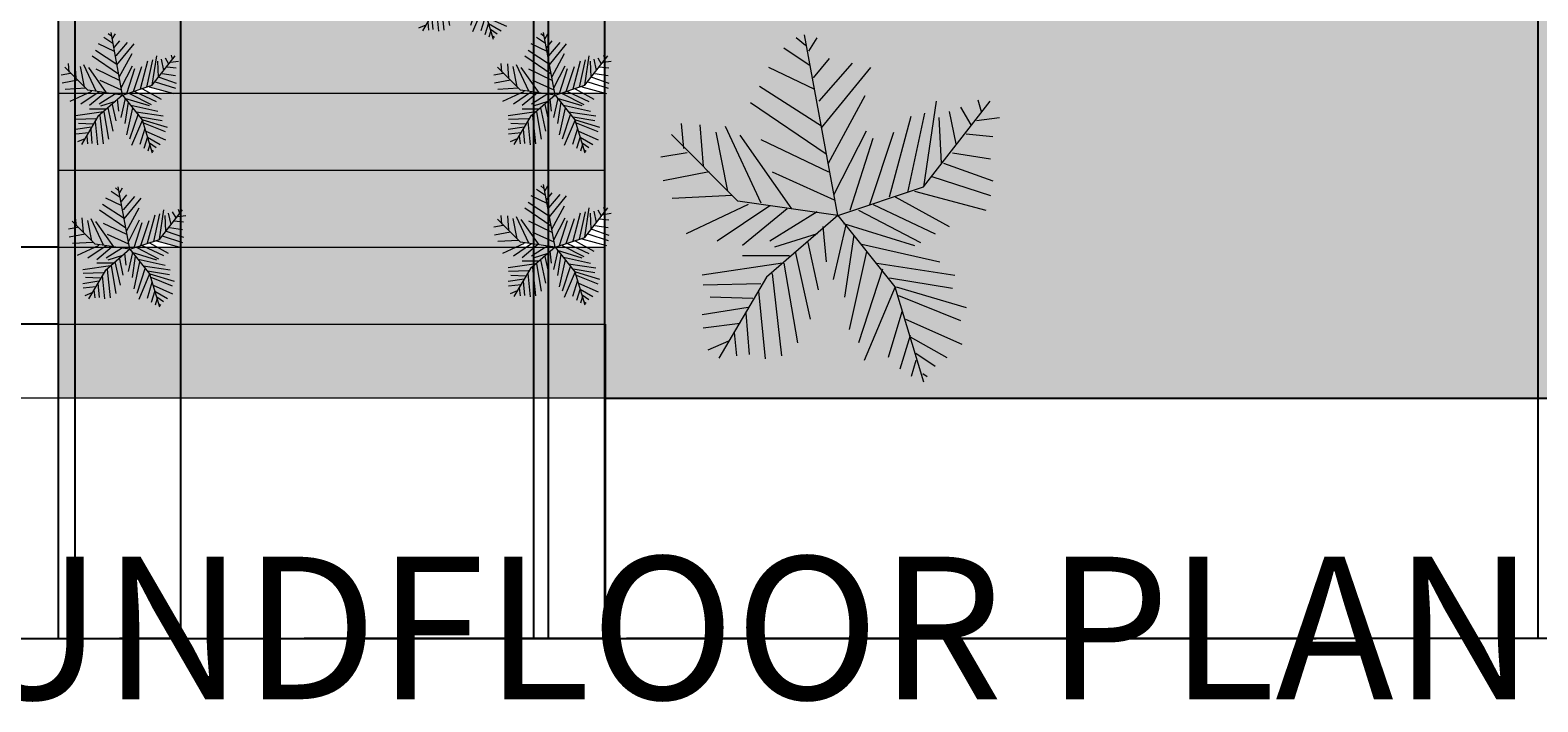
# Model space of a CAD drawing. Units: millimetres. Extents: x -229 to 16545, y -10488 to 4272.
# Tile 6 of 29: x 5862 to 12015, y -10488 to -7746. Entities that reach past the tile are written whole.
import ezdxf

# ---------------------------------------------------------------- set-up
doc = ezdxf.new("R2010")
doc.units = ezdxf.units.MM
for name, color, linetype, lineweight in [('A-ANNO-DIMS', 2, 'Continuous', 18), ('A-ANNO-TEXT', 7, 'Continuous', 25), ('A-FLOR-STRS', 7, 'Continuous', 18), ('L-PLNT-TREE', 80, 'Continuous', 18), ('L-PVMT', 7, 'Continuous', 18)]:
    doc.layers.add(name, color=color, linetype=linetype, lineweight=lineweight)
doc.layers.add('A-FLOR-STRS-PATT', color=51, linetype='Continuous', lineweight=13, true_color=0xf8f6b0)
doc.layers.add('L-PLNT-PATT', color=116, linetype='Continuous', lineweight=13, true_color=0x136734)
doc.styles.get("Standard").update_dxf_attribs({"font": 'arial.ttf'})
doc.dimstyles.get("Standard").update_dxf_attribs({"dimtxt": 0.18, "dimasz": 0.18, "dimexe": 0.18, "dimexo": 0.0625, "dimgap": 0.09, "dimtad": 0, "dimtih": 1, "dimtoh": 1, "dimdec": 4, "dimzin": 0, "dimdsep": 46, "dimtxsty": 'Standard', "dimcen": 0.09, "dimadec": 0, "dimazin": 0, "dimtfac": 1, "dimtdec": 4, "dimtofl": 0, "dimtmove": 0, "dimatfit": 3, "dimfxl": 1, "dimtolj": 1, "dimtzin": 0, "dimarcsym": 0})

# ---------------------------------------------------------------- blocks, each defined once
blk = doc.blocks.new('*U18')
for p, q in [((-8.737, 47.138), (-17.069, 52.711)), ((-10.186, 53.64), (-13.084, 55.962)), ((0, 0), (-10.5, 57)), ((-9.099, 51.782), (-6.563, 55.962)), ((-7.65, 43.423), (-2.578, 49.46)), ((-5.839, 35.992), (4.667, 48.067)), ((-7.288, 39.707), (-21.778, 46.673)), ((-5.114, 27.632), (10.463, 46.673)), ((-5.114, 28.097), (-24.676, 40.636)), ((-3.665, 19.273), (-27.574, 35.527)), ((-2.941, 16.486), (8.652, 37.85)), ((27, 9), (48, 36)), ((27.127, 9.056), (31.112, 35.992)), ((38.719, 34.134), (41.979, 28.561)), ((44.153, 36.456), (45.239, 32.741)), ((-48.585, 21.131), (-49.309, 29.026)), ((-43.513, 28.561), (-42.427, 15.558)), ((16.259, 5.805), (23.142, 31.348)), ((22.055, 7.198), (27.489, 32.277)), ((31.836, 30.883), (32.561, 16.486)), ((35.096, 32.741), (37.27, 22.524)), ((43.791, 29.954), (51.036, 30.883)), ((-31.5, 4.5), (-52.5, 25.5)), ((-38.442, 26.239), (-34.819, 7.663)), ((-35.544, 28.097), (-24.314, 3.947)), ((-14.533, 2.09), (-30.834, 25.31)), ((-24.314, 23.917), (-2.941, 13.7)), ((-1.129, 6.734), (9.014, 26.704)), ((3.942, 1.625), (11.187, 24.381)), ((10.101, 3.483), (17.708, 26.239)), ((40.53, 25.775), (48.862, 24.846)), ((-47.498, 19.737), (-55.83, 18.344)), ((36.183, 19.737), (48.137, 17.88)), ((33.285, 16.486), (48.862, 10.913)), ((-40.615, 13.7), (-55.105, 10.913)), ((-20.691, 13.7), (-1.129, 4.876)), ((29.662, 12.307), (48.137, 6.269)), ((-33.37, 6.269), (-52.207, 5.34)), ((0, 0), (27, 9)), ((18.07, 5.805), (35.096, -3.483)), ((24.229, 7.663), (46.688, 1.625)), ((-28.299, 3.483), (-47.86, -5.805)), ((-21.416, 3.018), (-38.079, -8.128)), ((0, 0), (-31.5, 4.5)), ((-15.982, 2.09), (-30.11, -9.521)), ((0, 0), (-22.5, -19.5)), ((-6.563, 1.161), (-21.416, -8.128)), ((0, 0), (18, -22.5)), ((6.478, 1.625), (26.04, -8.592)), ((11.187, 3.483), (30.749, -5.805)), ((-4.752, -3.483), (-3.665, -14.629)), ((2.493, -3.019), (-1.491, -20.202)), ((1.769, -2.555), (24.229, -9.521)), ((-6.563, -5.805), (-19.967, -9.985)), ((-9.461, -8.592), (-6.201, -23.453)), ((5.029, -6.27), (2.131, -25.775)), ((7.565, -9.056), (32.198, -14.629)), ((-15.257, -12.772), (-30.11, -12.772)), ((-13.446, -11.378), (-8.737, -32.741)), ((9.014, -11.378), (3.58, -35.992)), ((-17.431, -15.094), (-42.789, -18.809)), ((-20.691, -18.345), (-17.793, -44.352)), ((-17.069, -15.094), (-12.721, -40.172)), ((14.085, -16.951), (6.478, -40.172)), ((12.274, -15.094), (36.907, -18.809)), ((-24.314, -21.596), (-42.427, -22.06)), ((-22.5, -19.5), (-37.5, -45)), ((18.07, -22.524), (8.289, -45.745)), ((16.259, -19.738), (36.183, -22.989)), ((18, -22.5), (27, -52.5)), ((18.433, -22.524), (40.53, -29.026)), ((-26.849, -26.24), (-40.253, -25.775)), ((-25.038, -23.918), (-22.865, -45.281)), ((19.157, -25.311), (38.719, -33.206)), ((-28.299, -29.026), (-42.789, -31.348)), ((-29.023, -30.884), (-27.936, -43.887)), ((20.244, -30.419), (15.897, -44.816)), ((21.331, -32.741), (39.081, -40.636)), ((-30.834, -34.135), (-42.427, -35.528)), ((-32.646, -36.921), (-31.921, -44.352)), ((22.78, -37.85), (19.519, -48.532)), ((-34.457, -39.708), (-40.978, -42.494)), ((22.78, -38.314), (34.372, -44.816)), ((24.591, -45.745), (23.142, -50.854)), ((24.591, -43.423), (30.749, -47.603)), ((26.764, -49.925), (28.213, -50.854))]:
    blk.add_line(p, q)
blk = doc.blocks.new('*D47')
at = {"layer": 'A-ANNO-DIMS', "color": 0, "lineweight": -2, "transparency": 16777216}
for p, q in [((912.1, -9248.3), (912.1, -10230.2)), ((15679.6, -9248.3), (15679.6, -10230.2)), ((912.2, -10230), (8295.4, -10230)), ((15679.4, -10230), (8296.3, -10230))]:
    blk.add_line(p, q, dxfattribs=at)
at = {"layer": 'A-ANNO-DIMS', "color": 0, "transparency": 16777216}
for points in [[(912.2, -10230), (912.2, -10230.1), (912.1, -10230)], [(15679.4, -10230), (15679.4, -10230.1), (15679.6, -10230)]]:
    blk.add_solid(points, dxfattribs=at)
at = {"layer": 'Defpoints', "color": 0, "transparency": 16777216}
for p in [(912.1, -9248.3), (15679.6, -9248.3), (15679.6, -10230)]:
    blk.add_point(p, dxfattribs=at)
at = {"layer": 'A-ANNO-DIMS', "color": 0, "transparency": 16777216, "insert": (8295.8, -10230), "char_height": 0.18, "attachment_point": 5}
blk.add_mtext('\\A1;14768', dxfattribs=at)
blk = doc.blocks.new('*D59')
at = {"layer": 'A-ANNO-DIMS', "color": 0, "lineweight": -2, "transparency": 16777216}
for p, q in [((5975.9, -8946.8), (5975.9, -10230.2)), ((8209.2, -8946.8), (8209.2, -10230.2)), ((5976.1, -10230), (7092.1, -10230)), ((8209, -10230), (7093, -10230))]:
    blk.add_line(p, q, dxfattribs=at)
at = {"layer": 'A-ANNO-DIMS', "color": 0, "transparency": 16777216}
for points in [[(5976.1, -10230), (5976.1, -10230.1), (5975.9, -10230)], [(8209, -10230), (8209, -10230.1), (8209.2, -10230)]]:
    blk.add_solid(points, dxfattribs=at)
at = {"layer": 'Defpoints', "color": 0, "transparency": 16777216}
for p in [(5975.9, -8946.8), (8209.2, -8946.8), (8209.2, -10230)]:
    blk.add_point(p, dxfattribs=at)
at = {"layer": 'A-ANNO-DIMS', "color": 0, "transparency": 16777216, "insert": (7092.5, -10230), "char_height": 0.18, "attachment_point": 5}
blk.add_mtext('\\A1;2233.2', dxfattribs=at)
blk = doc.blocks.new('*D60')
at = {"layer": 'A-ANNO-DIMS', "color": 0, "lineweight": -2, "transparency": 16777216}
for p, q in [((8205.9, -7438.3), (8205.9, -10230.2)), ((14015.9, -7438.3), (14015.9, -10230.2)), ((8206.1, -10230), (11110.6, -10230)), ((14015.8, -10230), (11111.3, -10230))]:
    blk.add_line(p, q, dxfattribs=at)
at = {"layer": 'A-ANNO-DIMS', "color": 0, "transparency": 16777216}
for points in [[(8206.1, -10230), (8206.1, -10230.1), (8205.9, -10230)], [(14015.8, -10230), (14015.8, -10230.1), (14015.9, -10230)]]:
    blk.add_solid(points, dxfattribs=at)
at = {"layer": 'Defpoints', "color": 0, "transparency": 16777216}
for p in [(8205.9, -7438.3), (14015.9, -7438.3), (14015.9, -10230)]:
    blk.add_point(p, dxfattribs=at)
at = {"layer": 'A-ANNO-DIMS', "color": 0, "transparency": 16777216, "insert": (11110.9, -10230), "char_height": 0.18, "attachment_point": 5}
blk.add_mtext('\\A1;5810', dxfattribs=at)
blk = doc.blocks.new('*D63')
at = {"layer": 'A-ANNO-DIMS', "color": 0, "lineweight": -2, "transparency": 16777216}
for p, q in [((6475.9, -5438.3), (6475.9, -10230.2)), ((7975.9, -5438.3), (7975.9, -10230.2)), ((6476.1, -10230), (7225.6, -10230)), ((7975.8, -10230), (7226.3, -10230))]:
    blk.add_line(p, q, dxfattribs=at)
at = {"layer": 'A-ANNO-DIMS', "color": 0, "transparency": 16777216}
for points in [[(6476.1, -10230), (6476.1, -10230.1), (6475.9, -10230)], [(7975.8, -10230), (7975.8, -10230.1), (7975.9, -10230)]]:
    blk.add_solid(points, dxfattribs=at)
at = {"layer": 'Defpoints', "color": 0, "transparency": 16777216}
for p in [(6475.9, -5438.3), (7975.9, -5438.3), (7975.9, -10230)]:
    blk.add_point(p, dxfattribs=at)
at = {"layer": 'A-ANNO-DIMS', "color": 0, "transparency": 16777216, "insert": (7225.9, -10230), "char_height": 0.18, "attachment_point": 5}
blk.add_mtext('\\A1;1500', dxfattribs=at)
blk = doc.blocks.new('*D79')
at = {"layer": 'A-ANNO-DIMS', "color": 0, "lineweight": -2, "transparency": 16777216}
for p, q in [((8206, -7668.3), (16544.5, -7668.3)), ((16544.3, -7668.5), (16544.3, -8458.1)), ((16544.3, -9248.1), (16544.3, -8458.5)), ((8209.2, -9248.3), (16544.5, -9248.3))]:
    blk.add_line(p, q, dxfattribs=at)
at = {"layer": 'A-ANNO-DIMS', "color": 0, "transparency": 16777216}
for points in [[(16544.3, -7668.5), (16544.4, -7668.5), (16544.3, -7668.3)], [(16544.3, -9248.1), (16544.4, -9248.1), (16544.3, -9248.3)]]:
    blk.add_solid(points, dxfattribs=at)
at = {"layer": 'Defpoints', "color": 0, "transparency": 16777216}
for p in [(8205.9, -7668.3), (8209.2, -9248.3), (16544.3, -9248.3)]:
    blk.add_point(p, dxfattribs=at)
at = {"layer": 'A-ANNO-DIMS', "color": 0, "transparency": 16777216, "insert": (16544.3, -8458.3), "char_height": 0.18, "attachment_point": 5}
blk.add_mtext('\\A1;1580', dxfattribs=at)
blk = doc.blocks.new('*D80')
at = {"layer": 'A-ANNO-DIMS', "color": 0, "lineweight": -2, "transparency": 16777216}
for p, q in [((6043.9, -7218.3), (6043.9, -10230.2)), ((7916.5, -7218.3), (7916.5, -10230.2)), ((6044, -10230), (6979.7, -10230)), ((7916.3, -10230), (6980.6, -10230))]:
    blk.add_line(p, q, dxfattribs=at)
at = {"layer": 'A-ANNO-DIMS', "color": 0, "transparency": 16777216}
for points in [[(6044, -10230), (6044, -10230.1), (6043.9, -10230)], [(7916.3, -10230), (7916.3, -10230.1), (7916.5, -10230)]]:
    blk.add_solid(points, dxfattribs=at)
at = {"layer": 'Defpoints', "color": 0, "transparency": 16777216}
for p in [(6043.9, -7218.3), (7916.5, -7218.3), (7916.5, -10230)]:
    blk.add_point(p, dxfattribs=at)
at = {"layer": 'A-ANNO-DIMS', "color": 0, "transparency": 16777216, "insert": (6980.2, -10230), "char_height": 0.18, "attachment_point": 5}
blk.add_mtext('\\A1;1872.6', dxfattribs=at)
blk = doc.blocks.new('*D86')
at = {"layer": 'A-ANNO-DIMS', "color": 0, "lineweight": -2, "transparency": 16777216}
for p, q in [((8205.9, -5438.3), (8205.9, -10230.2)), ((12015.2, -5438.3), (12015.2, -10230.2)), ((8206.1, -10230), (10110.2, -10230)), ((12015, -10230), (10110.9, -10230))]:
    blk.add_line(p, q, dxfattribs=at)
at = {"layer": 'A-ANNO-DIMS', "color": 0, "transparency": 16777216}
for points in [[(8206.1, -10230), (8206.1, -10230.1), (8205.9, -10230)], [(12015, -10230), (12015, -10230.1), (12015.2, -10230)]]:
    blk.add_solid(points, dxfattribs=at)
at = {"layer": 'Defpoints', "color": 0, "transparency": 16777216}
for p in [(8205.9, -5438.3), (12015.2, -5438.3), (8205.9, -10230)]:
    blk.add_point(p, dxfattribs=at)
at = {"layer": 'A-ANNO-DIMS', "color": 0, "transparency": 16777216, "insert": (10110.6, -10230), "char_height": 0.18, "attachment_point": 5}
blk.add_mtext('\\A1;3809', dxfattribs=at)
blk = doc.blocks.new('*D90')
at = {"layer": 'A-ANNO-DIMS', "color": 0, "lineweight": -2, "transparency": 16777216}
for p, q in [((5975.9, -5438.3), (5975.9, -10230.2)), ((6475.9, -5438.3), (6475.9, -10230.2)), ((5976.1, -10230), (6225.6, -10230)), ((6475.8, -10230), (6226.2, -10230))]:
    blk.add_line(p, q, dxfattribs=at)
at = {"layer": 'A-ANNO-DIMS', "color": 0, "transparency": 16777216}
for points in [[(5976.1, -10230), (5976.1, -10230.1), (5975.9, -10230)], [(6475.8, -10230), (6475.8, -10230.1), (6475.9, -10230)]]:
    blk.add_solid(points, dxfattribs=at)
at = {"layer": 'Defpoints', "color": 0, "transparency": 16777216}
for p in [(5975.9, -5438.3), (6475.9, -5438.3), (6475.9, -10230)]:
    blk.add_point(p, dxfattribs=at)
at = {"layer": 'A-ANNO-DIMS', "color": 0, "transparency": 16777216, "insert": (6225.9, -10230), "char_height": 0.18, "attachment_point": 5}
blk.add_mtext('\\A1;500', dxfattribs=at)
blk = doc.blocks.new('*D98')
at = {"layer": 'A-ANNO-DIMS', "color": 0, "lineweight": -2, "transparency": 16777216}
for p, q in [((5975.9, -8632.3), (-228.8, -8632.3)), ((-228.7, -8632.5), (-228.7, -8789.3)), ((-228.7, -8946.6), (-228.7, -8789.7)), ((5975.9, -8946.8), (-228.8, -8946.8))]:
    blk.add_line(p, q, dxfattribs=at)
at = {"layer": 'A-ANNO-DIMS', "color": 0, "transparency": 16777216}
for points in [[(-228.7, -8632.5), (-228.6, -8632.5), (-228.7, -8632.3)], [(-228.7, -8946.6), (-228.6, -8946.6), (-228.7, -8946.8)]]:
    blk.add_solid(points, dxfattribs=at)
at = {"layer": 'Defpoints', "color": 0, "transparency": 16777216}
for p in [(-228.7, -8632.3), (5975.9, -8632.3), (5975.9, -8946.8)]:
    blk.add_point(p, dxfattribs=at)
at = {"layer": 'A-ANNO-DIMS', "color": 0, "transparency": 16777216, "insert": (-228.7, -8789.5), "char_height": 0.18, "attachment_point": 5}
blk.add_mtext('\\A1;314.45', dxfattribs=at)

msp = doc.modelspace()

# ---------------------------------------------------------------- hatches: boundary and pattern name
at = {"layer": 'A-FLOR-STRS-PATT', "transparency": 33554615}
h = msp.add_hatch(color=256, dxfattribs=at)
h.dxf.hatch_style = 1
h.paths.add_polyline_path([(8209.16, -7668.272), (5975.933, -7668.272), (5975.933, -8003.395), (6096.954, -8003.395), (6116.245, -7994.236), (6180.362, -8003.395), (6237.45, -8003.395), (6215.763, -7885.666), (6217.195, -7886.584), (6216.164, -7887.844), (6237.45, -8003.395), (6264.12, -8003.395), (6359.981, -7971.442), (6384.971, -7939.312), (6384.84, -7936.715), (6386.523, -7937.317), (6360.638, -7970.597), (6360.54, -7971.255), (6344.488, -7976.606), (6444.134, -8003.395), (7862.582, -8003.395), (7881.873, -7994.236), (7945.991, -8003.395), (8003.078, -8003.395), (7981.391, -7885.666), (7982.823, -7886.584), (7981.793, -7887.844), (8003.078, -8003.395), (8029.748, -8003.395), (8125.609, -7971.442), (8150.599, -7939.312), (8150.468, -7936.715), (8152.151, -7937.317), (8209.16, -7864.019)])
h.paths.add_polyline_path([(6610.327, -7438.272), (6608.323, -7440.849), (6608.225, -7441.508), (6486.678, -7482.023), (6409.988, -7548.488), (6430.756, -7668.272), (6531.713, -7668.272), (6567.486, -7583.344), (6567.184, -7582.338), (6567.83, -7582.528), (6567.486, -7583.344), (6588.563, -7653.601), (6614.718, -7668.272), (7510.183, -7668.272), (7529.817, -7634.894), (7630.64, -7547.514), (7522.745, -7532.1), (7479.114, -7438.272)])
h.paths.add_polyline_path([(8205.933, -7438.272), (7805.227, -7438.272), (7752.285, -7506.34), (7752.188, -7506.998), (7630.64, -7547.514), (7570.616, -7599.535), (7585.768, -7668.272), (7703.261, -7668.272), (7711.448, -7648.835), (7711.146, -7647.829), (7780.622, -7668.272), (8205.933, -7668.272)])
h.paths.add_polyline_path([(6486.678, -7482.023), (6378.783, -7466.61), (6365.606, -7438.272), (5975.933, -7438.272), (5975.933, -7668.272), (6312.811, -7668.272), (6332.694, -7659.777), (6385.855, -7569.403)])
h.paths.add_polyline_path([(8004.621, -8011.771), (7945.991, -8003.395), (6264.12, -8003.395), (6238.993, -8011.771), (6162.303, -8078.236), (6162.466, -8079.176), (6160.964, -8079.396), (6238.993, -8011.771), (6180.362, -8003.395), (5975.933, -8003.395), (5975.933, -8317.848), (8209.16, -8317.848), (8209.16, -8003.395), (8029.748, -8003.395), (8004.621, -8011.771), (7927.931, -8078.236), (7928.094, -8079.176), (7926.592, -8079.396)])
h.paths.add_polyline_path([(6340.675, -8182.674), (6340.529, -8183.153), (6340.878, -8183.349)], flags=16)
h.paths.add_polyline_path([(8106.304, -8182.674), (8106.157, -8183.153), (8106.506, -8183.349)], flags=16)
h.paths.add_polyline_path([(7981.391, -8506.197), (7982.823, -8507.115), (7981.793, -8508.375), (8004.621, -8632.301), (8125.609, -8591.972), (8150.599, -8559.842), (8150.468, -8557.245), (8152.151, -8557.847), (8209.16, -8484.549), (8209.16, -8317.848), (5975.933, -8317.848), (5975.933, -8632.301), (6126.407, -8632.301), (6145.698, -8623.142), (6209.815, -8632.301), (6266.903, -8632.301), (6245.216, -8514.572), (6246.648, -8515.49), (6245.617, -8516.75), (6266.903, -8632.301), (6293.573, -8632.301), (6389.434, -8600.348), (6414.424, -8568.218), (6414.293, -8565.621), (6415.975, -8566.223), (6390.091, -8599.503), (6389.993, -8600.161), (6373.941, -8605.512), (6473.587, -8632.301), (7844.942, -8632.301), (7881.873, -8614.766), (8004.621, -8632.301)])
h.paths.add_polyline_path([(8004.621, -8632.301), (6293.573, -8632.301), (6268.446, -8640.677), (6191.756, -8707.142), (6191.919, -8708.082), (6190.417, -8708.302), (6268.446, -8640.677), (6209.815, -8632.301), (5975.933, -8632.301), (5975.933, -8946.754), (8209.16, -8946.754), (8209.16, -8632.301), (8004.621, -8632.301), (7927.931, -8698.766), (7928.094, -8699.706), (7926.592, -8699.926)])
h.paths.add_polyline_path([(6370.128, -8811.58), (6369.982, -8812.059), (6370.331, -8812.255)], flags=16)
h.paths.add_polyline_path([(8106.304, -8803.204), (8106.157, -8803.684), (8106.506, -8803.879)], flags=16)
h.paths.add_polyline_path([(8209.16, -8946.754), (5975.933, -8946.754), (5975.933, -9248.272), (8209.16, -9248.272)])
at = {"layer": 'L-PLNT-PATT'}
h = msp.add_hatch(dxfattribs=at)
h.set_pattern_fill('GRASS', color=256, scale=2)
h.set_pattern_definition([(90, (-8141.222, -13125.504), (-35.921024, 35.921024), [9.525, -62.31705]), (45, (-8141.22, -13125.504), (-35.92102, 35.92102), [9.525, -41.275]), (135, (-8141.22, -13125.504), (-35.92102, -35.92102), [9.525, -41.275])])
h.paths.add_polyline_path([(15679.607, 2251.728), (14387.79, 2251.728), (14387.79, -7668.272), (8209.16, -7668.272), (8209.16, -9248.272), (14015.933, -9248.272), (15679.607, -9248.272)])

# ---------------------------------------------------------------- linework, layer by layer
at = {"layer": 'A-FLOR-STRS'}
for p, q in [((8209.16, -9248.272), (8209.16, -7668.272)), ((5975.933, -8003.395), (8209.16, -8003.395)), ((5975.933, -8317.848), (8209.16, -8317.848)), ((5975.933, -8632.301), (8209.16, -8632.301)), ((5975.933, -8946.754), (8209.16, -8946.754))]:
    msp.add_line(p, q, dxfattribs=at)
at = {"layer": 'L-PVMT'}
for p, q in [((5975.933, -9248.272), (5975.933, -5438.272)), ((14015.933, -9248.272), (2015.933, -9248.272))]:
    msp.add_line(p, q, dxfattribs=at)

# ---------------------------------------------------------------- block references
at = {"layer": 'L-PLNT-TREE'}
for p, xscale, yscale, zscale in [((7630.64, -7547.514), 4.481031954380777, 4.481031954380777, 4.481031954380777), ((6238.993, -8011.771), 4.481031954380777, 4.481031954380777, 4.481031954380777), ((8004.621, -8011.771), 4.481031954380777, 4.481031954380777, 4.481031954380777), ((9158.177, -8502.371), 12.94000768461256, 12.94000768461256, 12.94000768461256), ((6268.446, -8640.677), 4.481031954380777, 4.481031954380777, 4.481031954380777), ((8004.621, -8632.301), 4.481031954380777, 4.481031954380777, 4.481031954380777)]:
    msp.add_blockref('*U18', p, dxfattribs=dict(at, xscale=xscale, yscale=yscale, zscale=zscale))

# ---------------------------------------------------------------- texts
at = {"layer": 'A-ANNO-TEXT'}
msp.add_text('GROUNDFLOOR PLAN', height=582.3252, dxfattribs=at).set_placement((3943.489, -10477.814))

# ---------------------------------------------------------------- dimensions: what is measured, and where the dimension line sits
at = {"layer": 'A-ANNO-DIMS'}
for base, p1, p2, override, picture, middle in [((6475.933, -10230.041), (5975.933, -5438.272), (6475.933, -5438.272), {"dimdec": 0, "dimlfac": 1, "dimrnd": 0, "dimzin": 0, "dimdsep": 46, "dimlunit": 2}, '*D90', (6225.933, -10230.041)), ((7975.933, -10230.041), (6475.933, -5438.272), (7975.933, -5438.272), {"dimdec": 0, "dimlfac": 1, "dimrnd": 0, "dimzin": 0, "dimdsep": 46, "dimlunit": 2}, '*D63', (7225.933, -10230.041)), ((8205.933, -10230.041), (12015.17, -5438.272), (8205.933, -5438.272), {"dimdec": 0, "dimlfac": 1, "dimrnd": 0, "dimzin": 0, "dimdsep": 46, "dimlunit": 2}, '*D86', (10110.551, -10230.041)), ((7916.467, -10230.041), (6043.864, -7218.272), (7916.467, -7218.272), {"dimdec": 1, "dimlfac": 1, "dimrnd": 0, "dimzin": 0, "dimdsep": 46, "dimlunit": 2}, '*D80', (6980.166, -10230.041)), ((14015.933, -10230.041), (8205.933, -7438.272), (14015.933, -7438.272), {"dimdec": 0, "dimlfac": 1, "dimrnd": 0, "dimzin": 0, "dimdsep": 46, "dimlunit": 2}, '*D60', (11110.933, -10230.041)), ((8209.16, -10230.041), (5975.933, -8946.754), (8209.16, -8946.754), {"dimdec": 1, "dimlfac": 1, "dimrnd": 0, "dimzin": 0, "dimdsep": 46, "dimlunit": 2}, '*D59', (7092.547, -10230.041)), ((15679.607, -10230.041), (912.052, -9248.272), (15679.607, -9248.272), {"dimdec": 0, "dimlfac": 1, "dimrnd": 0, "dimzin": 0, "dimdsep": 46, "dimlunit": 2}, '*D47', (8295.83, -10230.041))]:
    dim = msp.add_linear_dim(base=base, p1=p1, p2=p2, dimstyle='Standard', override=override, dxfattribs=at)
    dim.commit()
    dim.dimension.update_dxf_attribs({"geometry": picture, "text_midpoint": middle})
for base, p1, p2, override, picture, middle in [((16544.342, -9248.272), (8205.933, -7668.272), (8209.16, -9248.272), {"dimdec": 0, "dimlfac": 1, "dimrnd": 0, "dimzin": 0, "dimdsep": 46, "dimlunit": 2}, '*D79', (16544.342, -8458.272)), ((-228.657, -8632.301), (5975.933, -8946.754), (5975.933, -8632.301), {"dimdec": 2, "dimlfac": 1, "dimrnd": 0, "dimzin": 0, "dimdsep": 46, "dimlunit": 2}, '*D98', (-228.657, -8789.528))]:
    dim = msp.add_linear_dim(base=base, p1=p1, p2=p2, angle=90, dimstyle='Standard', override=override, dxfattribs=at)
    dim.commit()
    dim.dimension.update_dxf_attribs({"geometry": picture, "text_midpoint": middle})

doc.saveas('drawing.dxf')
